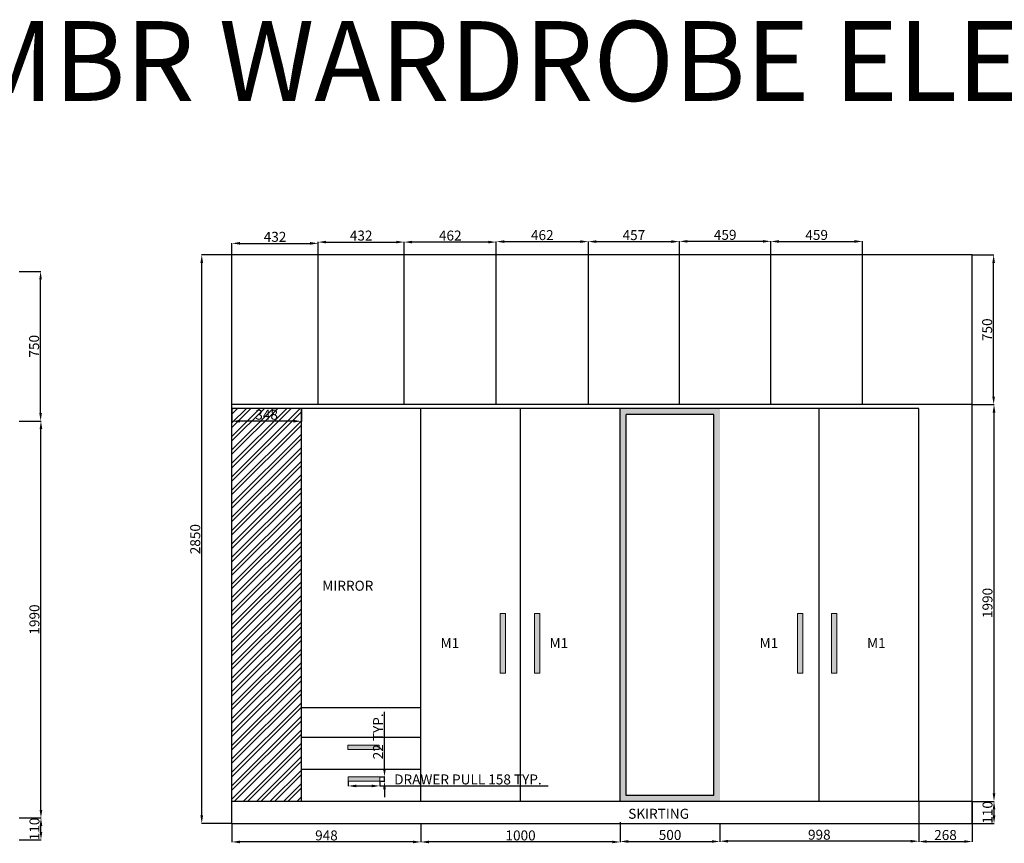
# Model space of a CAD drawing. Units: millimetres. Extents: x 46070 to 59439, y 6883 to 14761.
# Tile 3 of 5: x 49997 to 54938, y 10632 to 14761. Entities that reach past the tile are written whole.
import ezdxf

# ---------------------------------------------------------------- set-up
doc = ezdxf.new("R2010")
doc.units = ezdxf.units.MM
for name, color, linetype, lineweight in [('A-ANNO-DIMS', 2, 'Continuous', 18), ('A-ANNO-TEXT', 7, 'Continuous', 18), ('A-ELEV', 7, 'Continuous', 25), ('A-ELEV-PATT', 8, 'Continuous', 13), ('A-FURN-HDWR', 4, 'Continuous', 18)]:
    doc.layers.add(name, color=color, linetype=linetype, lineweight=lineweight)
doc.styles.get("Standard").update_dxf_attribs({"font": 'arial.ttf'})
doc.dimstyles.new('ISO-25', dxfattribs={"dimtxt": 50, "dimasz": 40, "dimexe": 1.25, "dimexo": 0.625, "dimtad": 1, "dimtxsty": 'Standard', "dimcen": 2.5, "dimadec": 0, "dimazin": 0, "dimtfac": 1, "dimtmove": 0, "dimatfit": 3, "dimfxl": 1, "dimarcsym": 0})

# ---------------------------------------------------------------- blocks, each defined once
blk = doc.blocks.new('*D1')
at = {"layer": 'A-ANNO-DIMS', "color": 0, "lineweight": -2, "transparency": 16777216}
for p, q in [((49995.3, 10759), (50105.5, 10759)), ((50104.2, 10689), (50104.2, 10719)), ((49995.3, 10649), (50105.5, 10649))]:
    blk.add_line(p, q, dxfattribs=at)
at = {"layer": 'A-ANNO-DIMS', "color": 0, "transparency": 16777216}
for points in [[(50097.5, 10719), (50110.9, 10719), (50104.2, 10759)], [(50097.5, 10689), (50110.9, 10689), (50104.2, 10649)]]:
    blk.add_solid(points, dxfattribs=at)
at = {"layer": 'Defpoints', "color": 0, "transparency": 16777216}
for p in [(49994.7, 10759), (50104.2, 10759), (49994.7, 10649)]:
    blk.add_point(p, dxfattribs=at)
at = {"layer": 'A-ANNO-DIMS', "color": 0, "transparency": 16777216, "insert": (50078.1, 10703.9), "char_height": 50, "attachment_point": 5, "rotation": 90}
blk.add_mtext('110', dxfattribs=at)
blk = doc.blocks.new('*D2')
at = {"layer": 'A-ANNO-DIMS', "color": 0, "lineweight": -2, "transparency": 16777216}
for p, q in [((49995.3, 12749), (50105.3, 12749)), ((50104.1, 10799), (50104.1, 12709)), ((49995.3, 10759), (50105.3, 10759))]:
    blk.add_line(p, q, dxfattribs=at)
at = {"layer": 'A-ANNO-DIMS', "color": 0, "transparency": 16777216}
for points in [[(50097.4, 12709), (50110.8, 12709), (50104.1, 12749)], [(50097.4, 10799), (50110.8, 10799), (50104.1, 10759)]]:
    blk.add_solid(points, dxfattribs=at)
at = {"layer": 'Defpoints', "color": 0, "transparency": 16777216}
for p in [(49994.7, 12749), (50104.1, 12749), (49994.7, 10759)]:
    blk.add_point(p, dxfattribs=at)
at = {"layer": 'A-ANNO-DIMS', "color": 0, "transparency": 16777216, "insert": (50077.9, 11754), "char_height": 50, "attachment_point": 5, "rotation": 90}
blk.add_mtext('1990', dxfattribs=at)
blk = doc.blocks.new('*D3')
at = {"layer": 'A-ANNO-DIMS', "color": 0, "lineweight": -2, "transparency": 16777216}
for p, q in [((49995.3, 13499), (50103.6, 13499)), ((50102.3, 12789), (50102.3, 13459)), ((49995.3, 12749), (50103.6, 12749))]:
    blk.add_line(p, q, dxfattribs=at)
at = {"layer": 'A-ANNO-DIMS', "color": 0, "transparency": 16777216}
for points in [[(50095.6, 13459), (50109, 13459), (50102.3, 13499)], [(50095.6, 12789), (50109, 12789), (50102.3, 12749)]]:
    blk.add_solid(points, dxfattribs=at)
at = {"layer": 'Defpoints', "color": 0, "transparency": 16777216}
for p in [(49994.7, 13499), (50102.3, 13499), (49994.7, 12749)]:
    blk.add_point(p, dxfattribs=at)
at = {"layer": 'A-ANNO-DIMS', "color": 0, "transparency": 16777216, "insert": (50076.2, 13124), "char_height": 50, "attachment_point": 5, "rotation": 90}
blk.add_mtext('750', dxfattribs=at)
blk = doc.blocks.new('*D24')
at = {"layer": 'A-ANNO-DIMS', "color": 0, "lineweight": -2, "transparency": 16777216}
for p, q in [((54777.2, 10841.9), (54887.4, 10841.9)), ((54886.1, 10771.9), (54886.1, 10801.9)), ((54777.2, 10731.9), (54887.4, 10731.9))]:
    blk.add_line(p, q, dxfattribs=at)
at = {"layer": 'A-ANNO-DIMS', "color": 0, "transparency": 16777216}
for points in [[(54879.4, 10801.9), (54892.8, 10801.9), (54886.1, 10841.9)], [(54879.4, 10771.9), (54892.8, 10771.9), (54886.1, 10731.9)]]:
    blk.add_solid(points, dxfattribs=at)
at = {"layer": 'Defpoints', "color": 0, "transparency": 16777216}
for p in [(54776.6, 10841.9), (54886.1, 10841.9), (54776.6, 10731.9)]:
    blk.add_point(p, dxfattribs=at)
at = {"layer": 'A-ANNO-DIMS', "color": 0, "transparency": 16777216, "insert": (54860, 10786.8), "char_height": 50, "attachment_point": 5, "rotation": 90}
blk.add_mtext('110', dxfattribs=at)
blk = doc.blocks.new('*D18')
at = {"layer": 'A-ANNO-DIMS', "color": 0, "lineweight": -2, "transparency": 16777216}
for p, q in [((54777.2, 12831.9), (54887.2, 12831.9)), ((54886, 10881.9), (54886, 12791.9)), ((54777.2, 10841.9), (54887.2, 10841.9))]:
    blk.add_line(p, q, dxfattribs=at)
at = {"layer": 'A-ANNO-DIMS', "color": 0, "transparency": 16777216}
for points in [[(54879.3, 12791.9), (54892.7, 12791.9), (54886, 12831.9)], [(54879.3, 10881.9), (54892.7, 10881.9), (54886, 10841.9)]]:
    blk.add_solid(points, dxfattribs=at)
at = {"layer": 'Defpoints', "color": 0, "transparency": 16777216}
for p in [(54776.6, 12831.9), (54886, 12831.9), (54776.6, 10841.9)]:
    blk.add_point(p, dxfattribs=at)
at = {"layer": 'A-ANNO-DIMS', "color": 0, "transparency": 16777216, "insert": (54859.8, 11836.9), "char_height": 50, "attachment_point": 5, "rotation": 90}
blk.add_mtext('1990', dxfattribs=at)
blk = doc.blocks.new('*D25')
at = {"layer": 'A-ANNO-DIMS', "color": 0, "lineweight": -2, "transparency": 16777216}
for p, q in [((54777.2, 13581.9), (54885.5, 13581.9)), ((54884.2, 12871.9), (54884.2, 13541.9)), ((54777.2, 12831.9), (54885.5, 12831.9))]:
    blk.add_line(p, q, dxfattribs=at)
at = {"layer": 'A-ANNO-DIMS', "color": 0, "transparency": 16777216}
for points in [[(54877.5, 13541.9), (54890.9, 13541.9), (54884.2, 13581.9)], [(54877.5, 12871.9), (54890.9, 12871.9), (54884.2, 12831.9)]]:
    blk.add_solid(points, dxfattribs=at)
at = {"layer": 'Defpoints', "color": 0, "transparency": 16777216}
for p in [(54776.6, 13581.9), (54884.2, 13581.9), (54776.6, 12831.9)]:
    blk.add_point(p, dxfattribs=at)
at = {"layer": 'A-ANNO-DIMS', "color": 0, "transparency": 16777216, "insert": (54858.1, 13206.9), "char_height": 50, "attachment_point": 5, "rotation": 90}
blk.add_mtext('750', dxfattribs=at)
blk = doc.blocks.new('*D19')
at = {"layer": 'A-ANNO-DIMS', "color": 0, "lineweight": -2, "transparency": 16777216}
for p, q in [((53510.6, 10731.3), (53510.6, 10641.2)), ((54508.6, 10731.3), (54508.6, 10641.2)), ((54468.6, 10642.5), (53550.6, 10642.5))]:
    blk.add_line(p, q, dxfattribs=at)
at = {"layer": 'A-ANNO-DIMS', "color": 0, "transparency": 16777216}
for points in [[(53550.6, 10649.1), (53550.6, 10635.8), (53510.6, 10642.5)], [(54468.6, 10649.1), (54468.6, 10635.8), (54508.6, 10642.5)]]:
    blk.add_solid(points, dxfattribs=at)
at = {"layer": 'Defpoints', "color": 0, "transparency": 16777216}
for p in [(53510.6, 10731.9), (54508.6, 10731.9), (53510.6, 10642.5)]:
    blk.add_point(p, dxfattribs=at)
at = {"layer": 'A-ANNO-DIMS', "color": 0, "transparency": 16777216, "insert": (54009.6, 10668.6), "char_height": 50, "attachment_point": 5}
blk.add_mtext('998', dxfattribs=at)
blk = doc.blocks.new('*D20')
at = {"layer": 'A-ANNO-DIMS', "color": 0, "lineweight": -2, "transparency": 16777216}
for p, q in [((53010.6, 10731.3), (53010.6, 10640)), ((53510.6, 10731.3), (53510.6, 10640)), ((53050.6, 10641.2), (53470.6, 10641.2))]:
    blk.add_line(p, q, dxfattribs=at)
at = {"layer": 'A-ANNO-DIMS', "color": 0, "transparency": 16777216}
for points in [[(53050.6, 10647.9), (53050.6, 10634.6), (53010.6, 10641.2)], [(53470.6, 10647.9), (53470.6, 10634.6), (53510.6, 10641.2)]]:
    blk.add_solid(points, dxfattribs=at)
at = {"layer": 'Defpoints', "color": 0, "transparency": 16777216}
for p in [(53010.6, 10731.9), (53510.6, 10731.9), (53510.6, 10641.2)]:
    blk.add_point(p, dxfattribs=at)
at = {"layer": 'A-ANNO-DIMS', "color": 0, "transparency": 16777216, "insert": (53260.6, 10667.4), "char_height": 50, "attachment_point": 5}
blk.add_mtext('500', dxfattribs=at)
blk = doc.blocks.new('*D28')
at = {"layer": 'A-ANNO-DIMS', "color": 0, "lineweight": -2, "transparency": 16777216}
for p, q in [((52388.6, 13582.5), (52388.6, 13649.9)), ((52428.6, 13648.7), (52810.6, 13648.7)), ((52850.6, 13582.5), (52850.6, 13649.9))]:
    blk.add_line(p, q, dxfattribs=at)
at = {"layer": 'A-ANNO-DIMS', "color": 0, "transparency": 16777216}
for points in [[(52428.6, 13655.4), (52428.6, 13642), (52388.6, 13648.7)], [(52810.6, 13655.4), (52810.6, 13642), (52850.6, 13648.7)]]:
    blk.add_solid(points, dxfattribs=at)
at = {"layer": 'Defpoints', "color": 0, "transparency": 16777216}
for p in [(52850.6, 13648.7), (52388.6, 13581.9), (52850.6, 13581.9)]:
    blk.add_point(p, dxfattribs=at)
at = {"layer": 'A-ANNO-DIMS', "color": 0, "transparency": 16777216, "insert": (52619.6, 13674.8), "char_height": 50, "attachment_point": 5}
blk.add_mtext('462', dxfattribs=at)
blk = doc.blocks.new('*D26')
at = {"layer": 'A-ANNO-DIMS', "color": 0, "lineweight": -2, "transparency": 16777216}
for p, q in [((51926.6, 13582.5), (51926.6, 13647.6)), ((52348.6, 13646.4), (51966.6, 13646.4)), ((52388.6, 13582.5), (52388.6, 13647.6))]:
    blk.add_line(p, q, dxfattribs=at)
at = {"layer": 'A-ANNO-DIMS', "color": 0, "transparency": 16777216}
for points in [[(51966.6, 13653), (51966.6, 13639.7), (51926.6, 13646.4)], [(52348.6, 13653), (52348.6, 13639.7), (52388.6, 13646.4)]]:
    blk.add_solid(points, dxfattribs=at)
at = {"layer": 'Defpoints', "color": 0, "transparency": 16777216}
for p in [(51926.6, 13646.4), (51926.6, 13581.9), (52388.6, 13581.9)]:
    blk.add_point(p, dxfattribs=at)
at = {"layer": 'A-ANNO-DIMS', "color": 0, "transparency": 16777216, "insert": (52157.6, 13672.5), "char_height": 50, "attachment_point": 5}
blk.add_mtext('462', dxfattribs=at)
blk = doc.blocks.new('*D21')
at = {"layer": 'A-ANNO-DIMS', "color": 0, "lineweight": -2, "transparency": 16777216}
for p, q in [((51494.6, 13582.5), (51494.6, 13647.6)), ((51534.6, 13646.4), (51886.6, 13646.4)), ((51926.6, 13582.5), (51926.6, 13647.6))]:
    blk.add_line(p, q, dxfattribs=at)
at = {"layer": 'A-ANNO-DIMS', "color": 0, "transparency": 16777216}
for points in [[(51534.6, 13653), (51534.6, 13639.7), (51494.6, 13646.4)], [(51886.6, 13653), (51886.6, 13639.7), (51926.6, 13646.4)]]:
    blk.add_solid(points, dxfattribs=at)
at = {"layer": 'Defpoints', "color": 0, "transparency": 16777216}
for p in [(51926.6, 13646.4), (51494.6, 13581.9), (51926.6, 13581.9)]:
    blk.add_point(p, dxfattribs=at)
at = {"layer": 'A-ANNO-DIMS', "color": 0, "transparency": 16777216, "insert": (51710.6, 13672.5), "char_height": 50, "attachment_point": 5}
blk.add_mtext('432', dxfattribs=at)
blk = doc.blocks.new('*D27')
at = {"layer": 'A-ANNO-DIMS', "color": 0, "lineweight": -2, "transparency": 16777216}
for p, q in [((51062.6, 13582.5), (51062.6, 13641.2)), ((51102.6, 13640), (51454.6, 13640)), ((51494.6, 13582.5), (51494.6, 13641.2))]:
    blk.add_line(p, q, dxfattribs=at)
at = {"layer": 'A-ANNO-DIMS', "color": 0, "transparency": 16777216}
for points in [[(51102.6, 13646.6), (51102.6, 13633.3), (51062.6, 13640)], [(51454.6, 13646.6), (51454.6, 13633.3), (51494.6, 13640)]]:
    blk.add_solid(points, dxfattribs=at)
at = {"layer": 'Defpoints', "color": 0, "transparency": 16777216}
for p in [(51494.6, 13640), (51062.6, 13581.9), (51494.6, 13581.9)]:
    blk.add_point(p, dxfattribs=at)
at = {"layer": 'A-ANNO-DIMS', "color": 0, "transparency": 16777216, "insert": (51278.6, 13666.1), "char_height": 50, "attachment_point": 5}
blk.add_mtext('432', dxfattribs=at)
blk = doc.blocks.new('*D22')
at = {"layer": 'A-ANNO-DIMS', "color": 0, "lineweight": -2, "transparency": 16777216}
for p, q in [((52010.6, 10731.3), (52010.6, 10637.5)), ((53010.6, 10738.7), (53010.6, 10637.5)), ((52970.6, 10638.7), (52050.6, 10638.7))]:
    blk.add_line(p, q, dxfattribs=at)
at = {"layer": 'A-ANNO-DIMS', "color": 0, "transparency": 16777216}
for points in [[(52050.6, 10645.4), (52050.6, 10632), (52010.6, 10638.7)], [(52970.6, 10645.4), (52970.6, 10632), (53010.6, 10638.7)]]:
    blk.add_solid(points, dxfattribs=at)
at = {"layer": 'Defpoints', "color": 0, "transparency": 16777216}
for p in [(52010.6, 10731.9), (53010.6, 10739.4), (52010.6, 10638.7)]:
    blk.add_point(p, dxfattribs=at)
at = {"layer": 'A-ANNO-DIMS', "color": 0, "transparency": 16777216, "insert": (52510.6, 10664.9), "char_height": 50, "attachment_point": 5}
blk.add_mtext('1000', dxfattribs=at)
blk = doc.blocks.new('*D23')
at = {"layer": 'A-ANNO-DIMS', "color": 0, "lineweight": -2, "transparency": 16777216}
for p, q in [((51062.6, 10731.3), (51062.6, 10637.6)), ((52010.6, 10731.3), (52010.6, 10637.6)), ((51970.6, 10638.8), (51102.6, 10638.8))]:
    blk.add_line(p, q, dxfattribs=at)
at = {"layer": 'A-ANNO-DIMS', "color": 0, "transparency": 16777216}
for points in [[(51102.6, 10645.5), (51102.6, 10632.1), (51062.6, 10638.8)], [(51970.6, 10645.5), (51970.6, 10632.1), (52010.6, 10638.8)]]:
    blk.add_solid(points, dxfattribs=at)
at = {"layer": 'Defpoints', "color": 0, "transparency": 16777216}
for p in [(51062.6, 10731.9), (52010.6, 10731.9), (51062.6, 10638.8)]:
    blk.add_point(p, dxfattribs=at)
at = {"layer": 'A-ANNO-DIMS', "color": 0, "transparency": 16777216, "insert": (51536.6, 10665), "char_height": 50, "attachment_point": 5}
blk.add_mtext('948', dxfattribs=at)
blk = doc.blocks.new('*D29')
at = {"layer": 'A-ANNO-DIMS', "color": 0, "lineweight": -2, "transparency": 16777216}
for p, q in [((54508.6, 10841.3), (54508.6, 10639.7)), ((54776.6, 10841.3), (54776.6, 10639.7)), ((54548.6, 10640.9), (54736.6, 10640.9))]:
    blk.add_line(p, q, dxfattribs=at)
at = {"layer": 'A-ANNO-DIMS', "color": 0, "transparency": 16777216}
for points in [[(54548.6, 10647.6), (54548.6, 10634.3), (54508.6, 10640.9)], [(54736.6, 10647.6), (54736.6, 10634.3), (54776.6, 10640.9)]]:
    blk.add_solid(points, dxfattribs=at)
at = {"layer": 'Defpoints', "color": 0, "transparency": 16777216}
for p in [(54508.6, 10841.9), (54776.6, 10841.9), (54776.6, 10640.9)]:
    blk.add_point(p, dxfattribs=at)
at = {"layer": 'A-ANNO-DIMS', "color": 0, "transparency": 16777216, "insert": (54642.6, 10667.1), "char_height": 50, "attachment_point": 5}
blk.add_mtext('268', dxfattribs=at)
blk = doc.blocks.new('*D30')
at = {"layer": 'A-ANNO-DIMS', "color": 0, "lineweight": -2, "transparency": 16777216}
for p, q in [((51062, 13581.9), (50909.6, 13581.9)), ((50910.9, 10771.9), (50910.9, 13541.9)), ((51062, 10731.9), (50909.6, 10731.9))]:
    blk.add_line(p, q, dxfattribs=at)
at = {"layer": 'A-ANNO-DIMS', "color": 0, "transparency": 16777216}
for points in [[(50904.2, 13541.9), (50917.5, 13541.9), (50910.9, 13581.9)], [(50904.2, 10771.9), (50917.5, 10771.9), (50910.9, 10731.9)]]:
    blk.add_solid(points, dxfattribs=at)
at = {"layer": 'Defpoints', "color": 0, "transparency": 16777216}
for p in [(50910.9, 13581.9), (51062.6, 13581.9), (51062.6, 10731.9)]:
    blk.add_point(p, dxfattribs=at)
at = {"layer": 'A-ANNO-DIMS', "color": 0, "transparency": 16777216, "insert": (50884.7, 12156.9), "char_height": 50, "attachment_point": 5, "rotation": 90}
blk.add_mtext('2850', dxfattribs=at)
blk = doc.blocks.new('*D31')
at = {"layer": 'A-ANNO-DIMS', "color": 0, "lineweight": -2, "transparency": 16777216}
for p, q in [((52850.6, 13582.5), (52850.6, 13649.9)), ((52890.6, 13648.7), (53267.6, 13648.7)), ((53307.6, 13582.5), (53307.6, 13649.9))]:
    blk.add_line(p, q, dxfattribs=at)
at = {"layer": 'A-ANNO-DIMS', "color": 0, "transparency": 16777216}
for points in [[(52890.6, 13655.4), (52890.6, 13642), (52850.6, 13648.7)], [(53267.6, 13655.4), (53267.6, 13642), (53307.6, 13648.7)]]:
    blk.add_solid(points, dxfattribs=at)
at = {"layer": 'Defpoints', "color": 0, "transparency": 16777216}
for p in [(53307.6, 13648.7), (52850.6, 13581.9), (53307.6, 13581.9)]:
    blk.add_point(p, dxfattribs=at)
at = {"layer": 'A-ANNO-DIMS', "color": 0, "transparency": 16777216, "insert": (53079.1, 13674.7), "char_height": 50, "attachment_point": 5}
blk.add_mtext('457', dxfattribs=at)
blk = doc.blocks.new('*D32')
at = {"layer": 'A-ANNO-DIMS', "color": 0, "lineweight": -2, "transparency": 16777216}
for p, q in [((53307.6, 13582.5), (53307.6, 13651.2)), ((53726.6, 13649.9), (53347.6, 13649.9)), ((53766.6, 13582.5), (53766.6, 13651.2))]:
    blk.add_line(p, q, dxfattribs=at)
at = {"layer": 'A-ANNO-DIMS', "color": 0, "transparency": 16777216}
for points in [[(53347.6, 13656.6), (53347.6, 13643.3), (53307.6, 13649.9)], [(53726.6, 13656.6), (53726.6, 13643.3), (53766.6, 13649.9)]]:
    blk.add_solid(points, dxfattribs=at)
at = {"layer": 'Defpoints', "color": 0, "transparency": 16777216}
for p in [(53307.6, 13649.9), (53307.6, 13581.9), (53766.6, 13581.9)]:
    blk.add_point(p, dxfattribs=at)
at = {"layer": 'A-ANNO-DIMS', "color": 0, "transparency": 16777216, "insert": (53537.1, 13676.1), "char_height": 50, "attachment_point": 5}
blk.add_mtext('459', dxfattribs=at)
blk = doc.blocks.new('*D33')
at = {"layer": 'A-ANNO-DIMS', "color": 0, "lineweight": -2, "transparency": 16777216}
for p, q in [((53766.6, 13582.5), (53766.6, 13650.7)), ((53806.6, 13649.4), (54185.6, 13649.4)), ((54225.6, 13582.5), (54225.6, 13650.7))]:
    blk.add_line(p, q, dxfattribs=at)
at = {"layer": 'A-ANNO-DIMS', "color": 0, "transparency": 16777216}
for points in [[(53806.6, 13656.1), (53806.6, 13642.8), (53766.6, 13649.4)], [(54185.6, 13656.1), (54185.6, 13642.8), (54225.6, 13649.4)]]:
    blk.add_solid(points, dxfattribs=at)
at = {"layer": 'Defpoints', "color": 0, "transparency": 16777216}
for p in [(54225.6, 13649.4), (53766.6, 13581.9), (54225.6, 13581.9)]:
    blk.add_point(p, dxfattribs=at)
at = {"layer": 'A-ANNO-DIMS', "color": 0, "transparency": 16777216, "insert": (53996.1, 13675.6), "char_height": 50, "attachment_point": 5}
blk.add_mtext('459', dxfattribs=at)
blk = doc.blocks.new('*D42')
at = {"layer": 'A-ANNO-DIMS', "color": 0, "lineweight": -2, "transparency": 16777216}
for p, q in [((51062.6, 12811.3), (51062.6, 12747.1)), ((51410.6, 12811.3), (51410.6, 12747.1)), ((51370.6, 12748.3), (51102.6, 12748.3))]:
    blk.add_line(p, q, dxfattribs=at)
at = {"layer": 'A-ANNO-DIMS', "color": 0, "transparency": 16777216}
for points in [[(51102.6, 12755), (51102.6, 12741.6), (51062.6, 12748.3)], [(51370.6, 12755), (51370.6, 12741.6), (51410.6, 12748.3)]]:
    blk.add_solid(points, dxfattribs=at)
at = {"layer": 'Defpoints', "color": 0, "transparency": 16777216}
for p in [(51062.6, 12811.9), (51410.6, 12811.9), (51062.6, 12748.3)]:
    blk.add_point(p, dxfattribs=at)
at = {"layer": 'A-ANNO-DIMS', "color": 0, "transparency": 16777216, "insert": (51236.6, 12774.5), "char_height": 50, "attachment_point": 5}
blk.add_mtext('348', dxfattribs=at)
blk = doc.blocks.new('HANDLE-BAR-300')
blk.add_lwpolyline([(0, 299.3), (26.9, 299.3), (26.9, 0), (0, 0)], close=True)
blk = doc.blocks.new('DRAWER-PULL-160')
blk.add_lwpolyline([(0, 22.3), (158.3, 22.3), (158.3, 0), (0, 0)], close=True)
blk = doc.blocks.new('*D104')
at = {"layer": 'A-ANNO-DIMS', "color": 0, "lineweight": -2, "transparency": 16777216}
for p, q in [((51645.7, 10942.7), (51645.7, 10918.3)), ((51685.7, 10919.5), (51764, 10919.5)), ((51804, 10942.7), (51804, 10918.3)), ((51804, 10919.5), (52649, 10919.5))]:
    blk.add_line(p, q, dxfattribs=at)
at = {"layer": 'A-ANNO-DIMS', "color": 0, "transparency": 16777216}
for points in [[(51685.7, 10926.2), (51685.7, 10912.9), (51645.7, 10919.5)], [(51764, 10926.2), (51764, 10912.9), (51804, 10919.5)]]:
    blk.add_solid(points, dxfattribs=at)
at = {"layer": 'Defpoints', "color": 0, "transparency": 16777216}
for p in [(51645.7, 10943.3), (51804, 10943.3), (51804, 10919.5)]:
    blk.add_point(p, dxfattribs=at)
at = {"layer": 'A-ANNO-DIMS', "color": 0, "transparency": 16777216, "insert": (52246.5, 10945.7), "char_height": 50, "attachment_point": 5}
blk.add_mtext('DRAWER PULL 158 TYP.', dxfattribs=at)
blk = doc.blocks.new('*D105')
at = {"layer": 'A-ANNO-DIMS', "color": 0, "lineweight": -2, "transparency": 16777216}
for p, q in [((51827.8, 11005.5), (51827.8, 11291)), ((51804.7, 10965.5), (51829, 10965.5)), ((51804.7, 10943.3), (51829, 10943.3)), ((51827.8, 10943.3), (51827.8, 10965.5)), ((51827.8, 10903.3), (51827.8, 10863.3))]:
    blk.add_line(p, q, dxfattribs=at)
at = {"layer": 'A-ANNO-DIMS', "color": 0, "transparency": 16777216}
for points in [[(51821.1, 11005.5), (51834.4, 11005.5), (51827.8, 10965.5)], [(51821.1, 10903.3), (51834.4, 10903.3), (51827.8, 10943.3)]]:
    blk.add_solid(points, dxfattribs=at)
at = {"layer": 'Defpoints', "color": 0, "transparency": 16777216}
for p in [(51804, 10965.5), (51804, 10943.3), (51827.8, 10965.5)]:
    blk.add_point(p, dxfattribs=at)
at = {"layer": 'A-ANNO-DIMS', "color": 0, "transparency": 16777216, "insert": (51802, 11168.3), "char_height": 50, "attachment_point": 5, "rotation": 90}
blk.add_mtext('22 TYP.', dxfattribs=at)

msp = doc.modelspace()

# ---------------------------------------------------------------- hatches: boundary and pattern name
at = {"layer": 'A-ELEV-PATT'}
h = msp.add_hatch(dxfattribs=at)
h.set_pattern_fill('ANSI32', color=256, scale=5)
h.paths.add_polyline_path([(51410.593, 12811.888), (51062.593, 12811.888), (51062.593, 10841.888), (51410.593, 10841.888), (51410.593, 11161.888)])
h = msp.add_hatch(color=256, dxfattribs=at)
h.dxf.hatch_style = 1
h.paths.add_polyline_path([(53510.593, 12811.888), (53010.593, 12811.888), (53010.593, 10841.888), (53510.593, 10841.888)])
h.paths.add_polyline_path([(53480.593, 10871.888), (53040.593, 10871.888), (53040.593, 12781.888), (53480.593, 12781.888)], flags=16)
h = msp.add_hatch(color=256, dxfattribs=at)
h.dxf.hatch_style = 1
h.paths.add_polyline_path([(52580.053, 11485.309), (52606.971, 11485.309), (52606.971, 11784.593), (52580.053, 11784.593)])
h.paths.add_polyline_path([(52408.226, 11485.309), (52435.144, 11485.309), (52435.144, 11784.593), (52408.226, 11784.593)])
h = msp.add_hatch(color=256, dxfattribs=at)
h.dxf.hatch_style = 1
h.paths.add_polyline_path([(54071.16, 11485.309), (54098.078, 11485.309), (54098.078, 11784.593), (54071.16, 11784.593)])
h.paths.add_polyline_path([(53899.333, 11485.309), (53926.251, 11485.309), (53926.251, 11784.593), (53899.333, 11784.593)])
h = msp.add_hatch(color=256, dxfattribs=at)
h.dxf.hatch_style = 1
h.paths.add_polyline_path([(51801.689, 11101.484), (51801.689, 11123.749), (51643.387, 11123.749), (51643.387, 11101.484)])
h.paths.add_polyline_path([(51804.034, 10943.28), (51804.034, 10965.545), (51645.731, 10965.545), (51645.731, 10943.28)])

# ---------------------------------------------------------------- linework, layer by layer
at = {"layer": 'A-ELEV'}
for p, q in [((51062.593, 10731.888), (51062.593, 13581.888)), ((54776.593, 13581.888), (51062.593, 13581.888)), ((51494.593, 12831.888), (51494.593, 13581.888)), ((51926.593, 12831.888), (51926.593, 13581.888)), ((52388.593, 12831.888), (52388.593, 13581.888)), ((52850.593, 12831.888), (52850.593, 13581.888)), ((53307.593, 12831.888), (53307.593, 13581.888)), ((53766.593, 12831.888), (53766.593, 13581.888)), ((54225.593, 12831.888), (54225.593, 13581.888)), ((54776.593, 10731.888), (54776.593, 13581.888)), ((54776.593, 12831.888), (51062.593, 12831.888)), ((54508.593, 12811.888), (51062.593, 12811.888)), ((51410.593, 11161.888), (51410.593, 12811.888)), ((52010.593, 10841.888), (52010.593, 12811.888)), ((52508.593, 12811.888), (52508.593, 10841.888)), ((53010.593, 10841.888), (53010.593, 12811.888)), ((54009.593, 10841.888), (54009.593, 12811.888)), ((54508.593, 10841.888), (54508.593, 12811.888)), ((53040.593, 10871.888), (53040.593, 12781.888)), ((53480.593, 12781.888), (53040.593, 12781.888)), ((53480.593, 10871.888), (53480.593, 12781.888)), ((52010.593, 11311.888), (51410.593, 11311.888)), ((51410.593, 10841.888), (51410.593, 11161.888)), ((52010.593, 11161.888), (51410.593, 11161.888)), ((52010.593, 11001.888), (51410.593, 11001.888)), ((53480.593, 10871.888), (53040.593, 10871.888)), ((54776.593, 10841.888), (51062.593, 10841.888)), ((51062.593, 10731.888), (54776.593, 10731.888))]:
    msp.add_line(p, q, dxfattribs=at)

# ---------------------------------------------------------------- block references
at = {"layer": 'A-FURN-HDWR'}
for name, p in [('HANDLE-BAR-300', (52408.225, 11485.309)), ('HANDLE-BAR-300', (52580.053, 11485.309)), ('HANDLE-BAR-300', (53899.332, 11485.309)), ('HANDLE-BAR-300', (54071.16, 11485.309)), ('DRAWER-PULL-160', (51643.387, 11101.484)), ('DRAWER-PULL-160', (51645.731, 10943.28))]:
    msp.add_blockref(name, p, dxfattribs=at)

# ---------------------------------------------------------------- texts
at = {"layer": 'A-ANNO-TEXT', "attachment_point": 1}
for s, width, insert, char_height in [('MBR WARDROBE ELEVATION', 11748.56084, (49726.408, 14754.198), 400), ('MIRROR', 502.17574, (51515.798, 11948.32), 50), ('M1', 502.17574, (52109.317, 11660.651), 50), ('M1', 502.17574, (52655.766, 11660.651), 50), ('M1', 502.17574, (53709.884, 11660.651), 50), ('M1', 502.17574, (54249.094, 11660.651), 50), ('SKIRTING ', 502.17574, (53050.727, 10805.014), 50)]:
    msp.add_mtext_dynamic_manual_height_columns(s, width=width, gutter_width=12.5, heights=[0], dxfattribs=dict(at, insert=insert, char_height=char_height))

# ---------------------------------------------------------------- dimensions: what is measured, and where the dimension line sits
at = {"layer": 'A-ANNO-DIMS'}
for base, p1, p2, picture, middle in [((51494.593, 13639.967), (51062.593, 13581.888), (51494.593, 13581.888), '*D27', (51278.593, 13666.138)), ((51926.593, 13646.358), (51494.593, 13581.888), (51926.593, 13581.888), '*D21', (51710.593, 13672.529)), ((51926.593, 13646.358), (52388.593, 13581.888), (51926.593, 13581.888), '*D26', (52157.593, 13672.512)), ((52850.593, 13648.687), (52388.593, 13581.888), (52850.593, 13581.888), '*D28', (52619.593, 13674.84)), ((53307.593, 13648.687), (52850.593, 13581.888), (53307.593, 13581.888), '*D31', (53079.093, 13674.738)), ((53307.593, 13649.937), (53766.593, 13581.888), (53307.593, 13581.888), '*D32', (53537.093, 13676.09)), ((54225.593, 13649.446), (53766.593, 13581.888), (54225.593, 13581.888), '*D33', (53996.093, 13675.599)), ((51062.593, 12748.301), (51410.593, 12811.888), (51062.593, 12811.888), '*D42', (51236.593, 12774.472)), ((54776.593, 10640.927), (54508.593, 10841.888), (54776.593, 10841.888), '*D29', (54642.593, 10667.081)), ((51062.593, 10638.801), (52010.593, 10731.888), (51062.593, 10731.888), '*D23', (51536.593, 10664.955)), ((52010.593, 10638.711), (53010.593, 10739.362), (52010.593, 10731.888), '*D22', (52510.593, 10664.865)), ((53510.593, 10641.225), (53010.593, 10731.888), (53510.593, 10731.888), '*D20', (53260.593, 10667.378)), ((53510.593, 10642.475), (54508.593, 10731.888), (53510.593, 10731.888), '*D19', (54009.593, 10668.628))]:
    dim = msp.add_linear_dim(base=base, p1=p1, p2=p2, dimstyle='ISO-25', override={"dimclrd": 0, "dimclre": 0, "dimclrt": 0}, dxfattribs=at)
    dim.commit()
    dim.dimension.update_dxf_attribs({"geometry": picture, "text_midpoint": middle})
for base, p1, p2, picture, middle in [((50910.866, 13581.888), (51062.593, 10731.888), (51062.593, 13581.888), '*D30', (50884.712, 12156.888)), ((54884.209, 13581.888), (54776.593, 12831.888), (54776.593, 13581.888), '*D25', (54858.056, 13206.888)), ((50102.311, 13499.028), (49994.695, 12749.028), (49994.695, 13499.028), '*D3', (50076.157, 13124.028))]:
    dim = msp.add_linear_dim(base=base, p1=p1, p2=p2, angle=90, dimstyle='ISO-25', override={"dimclrd": 0, "dimclre": 0, "dimclrt": 0}, dxfattribs=at)
    dim.commit()
    dim.dimension.update_dxf_attribs({"geometry": picture, "text_midpoint": middle})
for base, p1, p2, picture, middle in [((54885.988, 12831.888), (54776.593, 10841.888), (54776.593, 12831.888), '*D18', (54885.988, 11836.888)), ((50104.089, 12749.028), (49994.695, 10759.028), (49994.695, 12749.028), '*D2', (50104.089, 11754.028)), ((54886.111, 10841.888), (54776.593, 10731.888), (54776.593, 10841.888), '*D24', (54886.111, 10786.786)), ((50104.213, 10759.028), (49994.695, 10649.028), (49994.695, 10759.028), '*D1', (50104.213, 10703.926))]:
    dim = msp.add_linear_dim(base=base, p1=p1, p2=p2, angle=90, dimstyle='ISO-25', override={"dimclrd": 0, "dimclre": 0, "dimclrt": 0}, dxfattribs=at)
    dim.commit()
    dim.dimension.update_dxf_attribs({"geometry": picture, "text_midpoint": middle, "dimtype": 160})
dim = msp.add_linear_dim(base=(51827.779, 10965.545), p1=(51804.034, 10943.28), p2=(51804.034, 10965.545), angle=90, text='<> TYP.', dimstyle='ISO-25', override={"dimdec": 0, "dimrnd": 0, "dimzin": 0, "dimlunit": 2}, dxfattribs=at)
dim.commit()
dim.dimension.update_dxf_attribs({"geometry": '*D105', "text_midpoint": (51802.035, 11168.288)})
dim = msp.add_linear_dim(base=(51804.034, 10919.535), p1=(51645.731, 10943.28), p2=(51804.034, 10943.28), text='DRAWER PULL <> TYP.', dimstyle='ISO-25', override={"dimdec": 0, "dimrnd": 0, "dimzin": 0, "dimlunit": 2}, dxfattribs=at)
dim.commit()
dim.dimension.update_dxf_attribs({"geometry": '*D104', "text_midpoint": (52246.517, 10945.689)})

doc.saveas('drawing.dxf')
